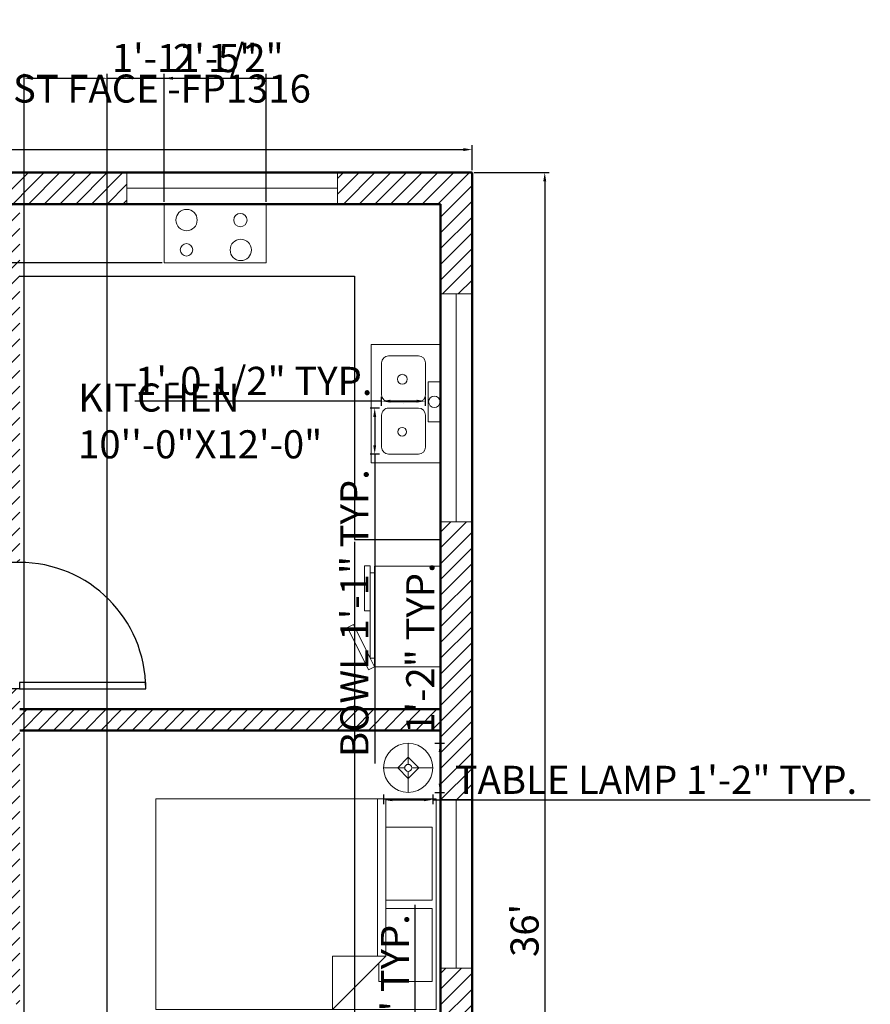
# Model space of a CAD drawing. Units: inches. Extents: x 1188 to 1681, y 1982 to 2608.
# Tile 4 of 4: x 1439 to 1681, y 2259 to 2540. Entities that reach past the tile are written whole.
import ezdxf

# ---------------------------------------------------------------- set-up
doc = ezdxf.new("R2010")
doc.units = ezdxf.units.IN
for name, color, linetype, lineweight in [('A-ANNO-DIMS', 2, 'Continuous', 18), ('A-ANNO-TEXT', 7, 'Continuous', 25), ('A-AREA-IDEN', 7, 'Continuous', 18), ('A-DOOR', 4, 'Continuous', 25), ('A-EQPM', 9, 'Continuous', 20), ('A-FLOR-CASE', 8, 'Continuous', 25), ('A-FLOR-FIXT', 9, 'Continuous', 18), ('A-FURN', 8, 'Continuous', 18), ('A-GLAZ', 4, 'Continuous', 20), ('A-WALL', 7, 'Continuous', 50), ('A-WALL-PATT', 8, 'Continuous', 13)]:
    doc.layers.add(name, color=color, linetype=linetype, lineweight=lineweight)
doc.styles.get("Standard").update_dxf_attribs({"font": 'arial.ttf'})
doc.dimstyles.new('ISO-25', dxfattribs={"dimtxt": 8, "dimasz": 2.5, "dimexe": 1.25, "dimexo": 0.625, "dimtad": 1, "dimdec": 1, "dimlunit": 4, "dimtxsty": 'Standard', "dimcen": 2.5, "dimadec": 0, "dimazin": 0, "dimtfac": 1, "dimtdec": 1, "dimtmove": 0, "dimatfit": 3, "dimfxl": 1, "dimarcsym": 0})

# ---------------------------------------------------------------- blocks, each defined once
blk = doc.blocks.new('*U5')
for p, q in [((0, 0), (0, 6)), ((36, 0), (36, 6))]:
    blk.add_line(p, q)
blk.add_lwpolyline([(0, 0), (0, -36), (1.75, -36), (1.75, 0)], close=True)
blk.add_arc((0, 0), 36, 270, 0)
blk = doc.blocks.new('Lamp - Table')
for p, q in [((0, 7), (0, 1)), ((0, 3), (-3, 0)), ((3, 0), (0, 3)), ((-1, 0), (-7, 0)), ((-3, 0), (0, -3)), ((0, -3), (3, 0)), ((1, 0), (7, 0)), ((0, -1), (0, -7))]:
    blk.add_line(p, q)
for radius in [7, 1]:
    blk.add_circle((0, 0), radius)
blk = doc.blocks.new('Bed - Queen')
for p, q in [((0, -80.00003), (0, 0)), ((0, 0), (59.99999, 0)), ((59.99999, 0), (59.99999, -80.00003)), ((7.99999, -1.2), (28.79998, -1.2)), ((7.99999, -14.4), (7.99999, -1.2)), ((28.79998, -1.2), (28.79998, -14.4)), ((31.19999, -1.2), (51.99999, -1.2)), ((31.19999, -14.4), (31.19999, -1.2)), ((51.99999, -1.2), (51.99999, -16.4)), ((0, -14.4), (44.8, -14.4)), ((44.8, -16.8), (0, -16.8)), ((59.99999, -29.6), (44.8, -14.4)), ((44.8, -14.4), (44.8, -29.6)), ((51.99999, -16.4), (46.79936, -16.4)), ((44.8, -29.6), (59.99999, -29.6)), ((59.99999, -80.00003), (0, -80.00003))]:
    blk.add_line(p, q)
blk = doc.blocks.new('*D13')
at = {"layer": 'A-ANNO-DIMS', "color": 0, "lineweight": -2, "transparency": 16777216}
for p, q in [((1568.34, 2496.41), (1589.68, 2496.41)), ((1588.43, 2493.91), (1588.43, 2066.91)), ((1568.34, 2064.41), (1589.68, 2064.41))]:
    blk.add_line(p, q, dxfattribs=at)
at = {"layer": 'A-ANNO-DIMS', "color": 0, "transparency": 16777216}
for points in [[(1588.02, 2493.91), (1588.85, 2493.91), (1588.43, 2496.41)], [(1588.02, 2066.91), (1588.85, 2066.91), (1588.43, 2064.41)]]:
    blk.add_solid(points, dxfattribs=at)
at = {"layer": 'Defpoints', "color": 0, "transparency": 16777216}
for p in [(1567.72, 2496.41), (1567.72, 2064.41), (1588.43, 2064.41)]:
    blk.add_point(p, dxfattribs=at)
at = {"layer": 'A-ANNO-DIMS', "color": 0, "transparency": 16777216, "insert": (1583.72, 2280.41), "char_height": 8, "attachment_point": 5, "rotation": 90}
blk.add_mtext("36'", dxfattribs=at)
blk = doc.blocks.new('*D14')
at = {"layer": 'A-ANNO-DIMS', "color": 0, "lineweight": -2, "transparency": 16777216}
for p, q in [((1231.72, 2497.04), (1231.72, 2504.18)), ((1567.72, 2497.04), (1567.72, 2504.18)), ((1234.22, 2502.93), (1565.22, 2502.93))]:
    blk.add_line(p, q, dxfattribs=at)
at = {"layer": 'A-ANNO-DIMS', "color": 0, "transparency": 16777216}
for points in [[(1234.22, 2503.35), (1234.22, 2502.52), (1231.72, 2502.93)], [(1565.22, 2503.35), (1565.22, 2502.52), (1567.72, 2502.93)]]:
    blk.add_solid(points, dxfattribs=at)
at = {"layer": 'Defpoints', "color": 0, "transparency": 16777216}
for p in [(1567.72, 2502.93), (1231.72, 2496.41), (1567.72, 2496.41)]:
    blk.add_point(p, dxfattribs=at)
at = {"layer": 'A-ANNO-DIMS', "color": 0, "transparency": 16777216, "insert": (1399.72, 2507.64), "char_height": 8, "attachment_point": 5}
blk.add_mtext("28'", dxfattribs=at)
blk = doc.blocks.new('WIN-60IN')
for p, q in [((0, 9), (0, 0)), ((60, 0), (60, 9)), ((60, 9), (60, 4.5)), ((60, 4.5), (0, 4.5)), ((0, 0), (60, 0))]:
    blk.add_line(p, q)
blk = doc.blocks.new('WIN-48IN')
for p, q in [((0, 9), (0, 0)), ((48, 0), (48, 9)), ((48, 9), (48, 4.5)), ((48, 4.5), (0, 4.5)), ((0, 0), (48, 0))]:
    blk.add_line(p, q)
blk = doc.blocks.new('SINK-BOWL')
for p, q in [((10.48, 13.11), (2, 13.11)), ((0, 11.11), (0, 2)), ((12.48, 2), (12.48, 11.11)), ((2, 0), (10.48, 0))]:
    blk.add_line(p, q)
for centre, start, end in [((2, 11.11), 90, 180), ((10.48, 11.11), 0, 90), ((2, 2), 180, 270), ((10.48, 2), 270, 0)]:
    blk.add_arc(centre, 2, start, end)
blk = doc.blocks.new('*D22')
at = {"layer": 'A-ANNO-DIMS', "color": 0, "lineweight": -2, "transparency": 16777216}
for p, q in [((1542.5, 2319.11), (1542.5, 2316.38)), ((1556.5, 2319.11), (1556.5, 2316.38)), ((1545, 2317.63), (1554, 2317.63)), ((1556.5, 2317.63), (1681.27, 2317.63))]:
    blk.add_line(p, q, dxfattribs=at)
at = {"layer": 'A-ANNO-DIMS', "color": 0, "transparency": 16777216}
for points in [[(1545, 2318.05), (1545, 2317.22), (1542.5, 2317.63)], [(1554, 2318.05), (1554, 2317.22), (1556.5, 2317.63)]]:
    blk.add_solid(points, dxfattribs=at)
at = {"layer": 'Defpoints', "color": 0, "transparency": 16777216}
for p in [(1542.5, 2319.73), (1556.5, 2319.73), (1556.5, 2317.63)]:
    blk.add_point(p, dxfattribs=at)
at = {"layer": 'A-ANNO-DIMS', "color": 0, "transparency": 16777216, "insert": (1620.14, 2322.28), "char_height": 8, "attachment_point": 5}
blk.add_mtext('TABLE LAMP 1\'-2" TYP.', dxfattribs=at)
blk = doc.blocks.new('*D23')
at = {"layer": 'A-ANNO-DIMS', "color": 0, "lineweight": -2, "transparency": 16777216}
for p, q in [((1558.6, 2333.73), (1558.6, 2385.5)), ((1557.13, 2333.73), (1559.85, 2333.73)), ((1558.6, 2322.23), (1558.6, 2331.23)), ((1557.13, 2319.73), (1559.85, 2319.73))]:
    blk.add_line(p, q, dxfattribs=at)
at = {"layer": 'A-ANNO-DIMS', "color": 0, "transparency": 16777216}
for points in [[(1558.19, 2331.23), (1559.02, 2331.23), (1558.6, 2333.73)], [(1558.19, 2322.23), (1559.02, 2322.23), (1558.6, 2319.73)]]:
    blk.add_solid(points, dxfattribs=at)
at = {"layer": 'Defpoints', "color": 0, "transparency": 16777216}
for p in [(1556.5, 2333.73), (1558.6, 2333.73), (1556.5, 2319.73)]:
    blk.add_point(p, dxfattribs=at)
at = {"layer": 'A-ANNO-DIMS', "color": 0, "transparency": 16777216, "insert": (1553.96, 2360.87), "char_height": 8, "attachment_point": 5, "rotation": 90}
blk.add_mtext('1\'-2" TYP.', dxfattribs=at)
blk = doc.blocks.new('*D26')
at = {"layer": 'A-ANNO-DIMS', "color": 0, "lineweight": -2, "transparency": 16777216}
for p, q in [((1551.52, 2182.72), (1551.52, 2287.7)), ((1558.09, 2182.72), (1550.27, 2182.72)), ((1551.52, 2137.22), (1551.52, 2180.22)), ((1558.09, 2134.72), (1550.27, 2134.72))]:
    blk.add_line(p, q, dxfattribs=at)
at = {"layer": 'A-ANNO-DIMS', "color": 0, "transparency": 16777216}
for points in [[(1551.1, 2180.22), (1551.93, 2180.22), (1551.52, 2182.72)], [(1551.1, 2137.22), (1551.93, 2137.22), (1551.52, 2134.72)]]:
    blk.add_solid(points, dxfattribs=at)
at = {"layer": 'Defpoints', "color": 0, "transparency": 16777216}
for p in [(1551.52, 2182.72), (1558.72, 2182.72), (1558.72, 2134.72)]:
    blk.add_point(p, dxfattribs=at)
at = {"layer": 'A-ANNO-DIMS', "color": 0, "transparency": 16777216, "insert": (1546.75, 2236.46), "char_height": 8, "attachment_point": 5, "rotation": 90}
blk.add_mtext('WINDOW 4\'-0" TYP.', dxfattribs=at)
blk = doc.blocks.new('*D36')
at = {"layer": 'A-ANNO-DIMS', "color": 0, "lineweight": -2, "transparency": 16777216}
for p, q in [((1541.29, 2429.27), (1538.7, 2429.27)), ((1539.95, 2426.77), (1539.95, 2418.66)), ((1541.29, 2416.16), (1538.7, 2416.16)), ((1539.95, 2416.16), (1539.95, 2327.98))]:
    blk.add_line(p, q, dxfattribs=at)
at = {"layer": 'A-ANNO-DIMS', "color": 0, "transparency": 16777216}
for points in [[(1539.54, 2426.77), (1540.37, 2426.77), (1539.95, 2429.27)], [(1539.54, 2418.66), (1540.37, 2418.66), (1539.95, 2416.16)]]:
    blk.add_solid(points, dxfattribs=at)
at = {"layer": 'Defpoints', "color": 0, "transparency": 16777216}
for p in [(1541.92, 2429.27), (1539.95, 2416.16), (1541.92, 2416.16)]:
    blk.add_point(p, dxfattribs=at)
at = {"layer": 'A-ANNO-DIMS', "color": 0, "transparency": 16777216, "insert": (1535.19, 2370.82), "char_height": 8, "attachment_point": 5, "rotation": 90}
blk.add_mtext('BOWL 1\'-1" TYP.', dxfattribs=at)
blk = doc.blocks.new('*D37')
at = {"layer": 'A-ANNO-DIMS', "color": 0, "lineweight": -2, "transparency": 16777216}
for p, q in [((1541.92, 2431.23), (1471.52, 2431.23)), ((1541.92, 2429.89), (1541.92, 2432.48)), ((1551.9, 2431.23), (1544.42, 2431.23)), ((1554.4, 2429.89), (1554.4, 2432.48))]:
    blk.add_line(p, q, dxfattribs=at)
at = {"layer": 'A-ANNO-DIMS', "color": 0, "transparency": 16777216}
for points in [[(1544.42, 2431.65), (1544.42, 2430.82), (1541.92, 2431.23)], [(1551.9, 2431.65), (1551.9, 2430.82), (1554.4, 2431.23)]]:
    blk.add_solid(points, dxfattribs=at)
at = {"layer": 'Defpoints', "color": 0, "transparency": 16777216}
for p in [(1541.92, 2431.23), (1541.92, 2429.27), (1554.4, 2429.27)]:
    blk.add_point(p, dxfattribs=at)
at = {"layer": 'A-ANNO-DIMS', "color": 0, "transparency": 16777216, "insert": (1505.47, 2435.99), "char_height": 8, "attachment_point": 5}
blk.add_mtext('1\'-0 1/2" TYP.', dxfattribs=at)
blk = doc.blocks.new('*D52')
at = {"layer": 'A-ANNO-DIMS', "color": 0, "lineweight": -2, "transparency": 16777216}
for p, q in [((1534.2, 2391.18), (1534.2, 1988.31)), ((1558.72, 2391.18), (1558.72, 1988.31)), ((1534.2, 1989.56), (1490.41, 1989.56)), ((1556.22, 1989.56), (1536.7, 1989.56))]:
    blk.add_line(p, q, dxfattribs=at)
at = {"layer": 'A-ANNO-DIMS', "color": 0, "transparency": 16777216}
for points in [[(1536.7, 1989.98), (1536.7, 1989.15), (1534.2, 1989.56)], [(1556.22, 1989.98), (1556.22, 1989.15), (1558.72, 1989.56)]]:
    blk.add_solid(points, dxfattribs=at)
at = {"layer": 'Defpoints', "color": 0, "transparency": 16777216}
for p in [(1534.2, 2391.81), (1558.72, 2391.81), (1534.2, 1989.56)]:
    blk.add_point(p, dxfattribs=at)
at = {"layer": 'A-ANNO-DIMS', "color": 0, "transparency": 16777216, "insert": (1511.06, 1994.33), "char_height": 8, "attachment_point": 5}
blk.add_mtext('2\'-0 1/2"', dxfattribs=at)
blk = doc.blocks.new('*D53')
at = {"layer": 'A-ANNO-DIMS', "color": 0, "lineweight": -2, "transparency": 16777216}
for p, q in [((1479.94, 2488.04), (1479.94, 2524.51)), ((1482.44, 2523.26), (1506.5, 2523.26)), ((1509, 2488.04), (1509, 2524.51))]:
    blk.add_line(p, q, dxfattribs=at)
at = {"layer": 'A-ANNO-DIMS', "color": 0, "transparency": 16777216}
for points in [[(1482.44, 2523.68), (1482.44, 2522.85), (1479.94, 2523.26)], [(1506.5, 2523.68), (1506.5, 2522.85), (1509, 2523.26)]]:
    blk.add_solid(points, dxfattribs=at)
at = {"layer": 'Defpoints', "color": 0, "transparency": 16777216}
for p in [(1509, 2523.26), (1479.94, 2487.41), (1509, 2487.41)]:
    blk.add_point(p, dxfattribs=at)
at = {"layer": 'A-ANNO-DIMS', "color": 0, "transparency": 16777216, "insert": (1494.47, 2527.97), "char_height": 8, "attachment_point": 5}
blk.add_mtext('2\'-5"', dxfattribs=at)
blk = doc.blocks.new('*D54')
at = {"layer": 'A-ANNO-DIMS', "color": 0, "lineweight": -2, "transparency": 16777216}
for p, q in [((1479.32, 2487.41), (1203.62, 2487.41)), ((1204.87, 2484.91), (1204.87, 2473.18)), ((1479.32, 2470.68), (1203.62, 2470.68)), ((1204.87, 2470.68), (1204.87, 2427.77))]:
    blk.add_line(p, q, dxfattribs=at)
at = {"layer": 'A-ANNO-DIMS', "color": 0, "transparency": 16777216}
for points in [[(1204.45, 2484.91), (1205.28, 2484.91), (1204.87, 2487.41)], [(1204.45, 2473.18), (1205.28, 2473.18), (1204.87, 2470.68)]]:
    blk.add_solid(points, dxfattribs=at)
at = {"layer": 'Defpoints', "color": 0, "transparency": 16777216}
for p in [(1479.94, 2487.41), (1204.87, 2470.68), (1479.94, 2470.68)]:
    blk.add_point(p, dxfattribs=at)
at = {"layer": 'A-ANNO-DIMS', "color": 0, "transparency": 16777216, "insert": (1200.11, 2447.98), "char_height": 8, "attachment_point": 5, "rotation": 90}
blk.add_mtext('1\'-4 1/2"', dxfattribs=at)
blk = doc.blocks.new('*D57')
at = {"layer": 'A-ANNO-DIMS', "color": 0, "lineweight": -2, "transparency": 16777216}
for p, q in [((1440.02, 2125.93), (1440.02, 2524.51)), ((1442.52, 2523.26), (1461.18, 2523.26)), ((1463.68, 2125.93), (1463.68, 2524.51)), ((1463.68, 2523.26), (1512.8, 2523.26))]:
    blk.add_line(p, q, dxfattribs=at)
at = {"layer": 'A-ANNO-DIMS', "color": 0, "transparency": 16777216}
for points in [[(1442.52, 2523.68), (1442.52, 2522.85), (1440.02, 2523.26)], [(1461.18, 2523.68), (1461.18, 2522.85), (1463.68, 2523.26)]]:
    blk.add_solid(points, dxfattribs=at)
at = {"layer": 'Defpoints', "color": 0, "transparency": 16777216}
for p in [(1463.68, 2523.26), (1440.02, 2125.31), (1463.68, 2125.31)]:
    blk.add_point(p, dxfattribs=at)
at = {"layer": 'A-ANNO-DIMS', "color": 0, "transparency": 16777216, "insert": (1489.49, 2528.03), "char_height": 8, "attachment_point": 5}
blk.add_mtext('1\'-11 1/2"', dxfattribs=at)

msp = doc.modelspace()

# ---------------------------------------------------------------- hatches: boundary and pattern name
at = {"layer": 'A-WALL-PATT', "transparency": 33554559}
h = msp.add_hatch(dxfattribs=at)
h.set_pattern_fill('ANSI31', color=256)
h.paths.add_polyline_path([(1390.99, 2496.41), (1231.72, 2496.41), (1231.72, 2452.82), (1240.72, 2452.82), (1240.72, 2487.41), (1390.99, 2487.41)])
h.paths.add_polyline_path([(1469.3, 2496.41), (1426.99, 2496.41), (1426.99, 2491.91), (1426.99, 2487.41), (1469.3, 2487.41)])
h.paths.add_polyline_path([(1378.72, 2487.41), (1372.72, 2487.41), (1372.72, 2404.84), (1372.72, 2343.41), (1367.48, 2343.41), (1367.48, 2337.41), (1378.72, 2337.41), (1378.72, 2391.41), (1387.67, 2391.41), (1387.67, 2397.41), (1378.72, 2397.41)])
h.paths.add_polyline_path([(1438.72, 2487.41), (1432.72, 2487.41), (1432.72, 2397.41), (1420.72, 2397.41), (1420.72, 2391.41), (1432.72, 2391.41), (1432.72, 2385.41), (1438.72, 2385.41)])
h.paths.add_polyline_path([(1240.72, 2392.82), (1236.22, 2392.82), (1231.72, 2392.82), (1231.72, 2323.77), (1240.72, 2323.77)])
h.paths.add_polyline_path([(1330.72, 2343.41), (1240.72, 2343.41), (1240.72, 2337.41), (1330.72, 2337.41)])
h.paths.add_polyline_path([(1558.72, 2343.41), (1438.72, 2343.41), (1438.72, 2349.29), (1438.64, 2349.29), (1432.72, 2349.29), (1432.72, 2259.41), (1438.72, 2259.41), (1438.72, 2337.41), (1558.72, 2337.41)])
h.paths.add_polyline_path([(1567.72, 2396.81), (1558.72, 2396.81), (1558.72, 2317.68), (1563.22, 2317.68), (1567.72, 2317.68)])
h.paths.add_polyline_path([(1567.72, 2496.41), (1529.3, 2496.41), (1529.3, 2491.91), (1529.3, 2487.41), (1558.72, 2487.41), (1558.72, 2461.81), (1567.72, 2461.81)])
h.paths.add_polyline_path([(1240.72, 2195.41), (1240.72, 2201.41), (1240.72, 2263.77), (1231.72, 2263.77), (1231.72, 2016.41), (1246.72, 2016.41), (1246.72, 2022.41), (1246.72, 2025.41), (1240.72, 2025.41)])
h.paths.add_polyline_path([(1391.72, 2211.41), (1397.72, 2211.41), (1397.72, 2217.41), (1385.72, 2217.41), (1385.72, 2163.41), (1366.72, 2163.41), (1366.72, 2157.41), (1385.72, 2157.41), (1385.72, 2073.41), (1391.72, 2073.41)])
h.paths.add_polyline_path([(1330.72, 2201.41), (1282.72, 2201.41), (1282.72, 2195.41), (1324.72, 2195.41), (1324.72, 2064.41), (1345.75, 2064.41), (1345.75, 2073.41), (1330.72, 2073.41), (1330.72, 2157.41), (1336.72, 2157.41), (1336.72, 2163.41), (1330.72, 2163.41)])
h.paths.add_polyline_path([(1558.72, 2217.41), (1438.72, 2217.41), (1438.72, 2223.26), (1432.72, 2223.26), (1432.72, 2217.41), (1427.72, 2217.41), (1427.72, 2211.41), (1432.72, 2211.41), (1558.72, 2211.41)])
h.paths.add_polyline_path([(1567.72, 2269.68), (1558.72, 2269.68), (1558.72, 2182.72), (1563.22, 2182.72), (1567.72, 2182.72)])
h.paths.add_polyline_path([(1567.72, 2134.72), (1558.72, 2134.72), (1558.72, 2073.41), (1497.85, 2073.41), (1497.85, 2068.91), (1497.85, 2064.41), (1567.72, 2064.41)])
h.paths.add_polyline_path([(1449.85, 2073.41), (1371.31, 2073.41), (1371.31, 2068.91), (1371.31, 2064.41), (1449.85, 2064.41)])
h.paths.add_polyline_path([(1333.72, 2064.41), (1324.72, 2064.41), (1324.72, 2025.41), (1313.9, 2025.41), (1313.9, 2016.41), (1333.72, 2016.41)])

# ---------------------------------------------------------------- linework, layer by layer
at = {"layer": 'A-EQPM'}
for p, q in [((1479.94, 2487.41), (1479.94, 2470.68)), ((1509, 2470.68), (1509, 2487.41)), ((1479.94, 2470.68), (1509, 2470.68)), ((1538.68, 2384.3), (1537, 2384.3)), ((1537, 2384.3), (1537, 2371.52)), ((1538.68, 2382.28), (1538.68, 2384.3)), ((1558.72, 2384.25), (1539.9, 2384.25)), ((1539.9, 2384.25), (1539.9, 2355.54)), ((1539.9, 2382.28), (1538.68, 2382.28)), ((1538.68, 2382.28), (1538.68, 2358.01)), ((1537, 2371.52), (1538.68, 2371.52)), ((1532.23, 2366.7), (1533.94, 2367.55)), ((1538.19, 2354.69), (1532.23, 2366.7)), ((1533.94, 2367.55), (1538.68, 2358.01)), ((1538.68, 2358.01), (1539.9, 2358.01)), ((1538.68, 2358.01), (1539.9, 2355.54)), ((1539.9, 2355.54), (1538.19, 2354.69)), ((1539.9, 2355.54), (1558.72, 2355.54))]:
    msp.add_line(p, q, dxfattribs=at)
for centre, radius in [((1486.29, 2482.85), 3.04), ((1501.64, 2482.85), 1.9), ((1486.29, 2474.35), 1.78), ((1501.77, 2474.35), 3.04)]:
    msp.add_circle(centre, radius, dxfattribs=at)
at = {"layer": 'A-FLOR-CASE'}
for p, q in [((1438.72, 2466.87), (1438.72, 2466.87)), ((1438.72, 2466.87), (1534.2, 2466.87)), ((1534.2, 2466.87), (1534.2, 2391.81)), ((1534.2, 2391.81), (1558.72, 2391.81))]:
    msp.add_line(p, q, dxfattribs=at)
at = {"layer": 'A-FLOR-FIXT'}
msp.add_line((1548.28, 2430.45), (1548.28, 2430.45), dxfattribs=at)
for points in [[(1558.72, 2447.35), (1538.96, 2447.35), (1538.96, 2413.68), (1558.72, 2413.68)], [(1555.18, 2436.76), (1558.72, 2436.76), (1558.72, 2425.38), (1555.18, 2425.38)]]:
    msp.add_lwpolyline(points, close=True, dxfattribs=at)
for centre, radius in [((1547.83, 2437.49), 1.4), ((1556.95, 2431.07), 1.63), ((1547.75, 2422.53), 1.23)]:
    msp.add_circle(centre, radius, dxfattribs=at)
at = {"layer": 'A-GLAZ'}
for p, q in [((1558.72, 2461.81), (1567.72, 2461.81)), ((1563.22, 2396.81), (1563.22, 2461.81)), ((1567.72, 2461.81), (1567.72, 2456.81)), ((1567.72, 2456.81), (1567.72, 2396.81)), ((1567.72, 2396.81), (1558.72, 2396.81)), ((1558.72, 2396.81), (1563.22, 2396.81))]:
    msp.add_line(p, q, dxfattribs=at)
at = {"layer": 'A-WALL'}
for p, q in [((1231.72, 2496.41), (1567.72, 2496.41)), ((1567.72, 2496.41), (1567.72, 2016.41)), ((1240.72, 2487.41), (1558.72, 2487.41)), ((1558.72, 2487.41), (1558.72, 2073.41)), ((1438.72, 2343.41), (1558.72, 2343.41)), ((1438.72, 2337.41), (1558.72, 2337.41))]:
    msp.add_line(p, q, dxfattribs=at)

# ---------------------------------------------------------------- block references
at = {"layer": 'A-DOOR', "rotation": 90}
msp.add_blockref('*U5', (1438.64, 2349.29), dxfattribs=at)
at = {"layer": 'A-FLOR-FIXT'}
msp.add_blockref('SINK-BOWL', (1541.92, 2431.05), dxfattribs=at)
at = {"layer": 'A-FLOR-FIXT', "rotation": 180}
msp.add_blockref('SINK-BOWL', (1554.4, 2429.27), dxfattribs=at)
at = {"layer": 'A-FURN'}
msp.add_blockref('Lamp - Table', (1549.5, 2326.73), dxfattribs=at)
at = {"layer": 'A-FURN', "rotation": 270}
msp.add_blockref('Bed - Queen', (1557.52, 2317.86), dxfattribs=at)
at = {"layer": 'A-GLAZ'}
msp.add_blockref('WIN-60IN', (1469.3, 2487.41), dxfattribs=at)
at = {"layer": 'A-GLAZ', "rotation": 89.99999999999909}
msp.add_blockref('WIN-48IN', (1567.72, 2269.68), dxfattribs=at)

# ---------------------------------------------------------------- texts
at = {"layer": 'A-ANNO-TEXT', "insert": (1239.94, 2524.33), "char_height": 8, "attachment_point": 1}
msp.add_mtext('28X40 (1120 SQ FT) HOUSSE PLAN - WEST FACE -FP1316', dxfattribs=at)
at = {"layer": 'A-AREA-IDEN', "insert": (1455.38, 2436.27), "char_height": 8, "attachment_point": 1}
msp.add_mtext('KITCHEN\\P10\'\'-0"X12\'-0"', dxfattribs=at)

# ---------------------------------------------------------------- dimensions: what is measured, and where the dimension line sits
at = {"layer": 'A-ANNO-DIMS'}
for base, p1, p2, override, picture, middle in [((1463.68, 2523.26), (1440.02, 2125.31), (1463.68, 2125.31), {"dimdec": 1, "dimlfac": 1, "dimrnd": 0, "dimzin": 1, "dimdsep": 46, "dimlunit": 4, "dimfrac": 2}, '*D57', (1489.49, 2528.03)), ((1509, 2523.26), (1479.94, 2487.41), (1509, 2487.41), {"dimdec": 1, "dimlfac": 1, "dimrnd": 0, "dimzin": 1, "dimdsep": 46, "dimlunit": 4, "dimfrac": 2}, '*D53', (1494.47, 2527.97)), ((1567.72, 2502.93), (1231.72, 2496.41), (1567.72, 2496.41), {"dimclrd": 0, "dimclre": 0, "dimclrt": 0}, '*D14', (1399.72, 2507.64)), ((1534.2, 1989.56), (1558.72, 2391.81), (1534.2, 2391.81), {"dimdec": 1, "dimlfac": 1, "dimrnd": 0, "dimzin": 1, "dimdsep": 46, "dimlunit": 4, "dimfrac": 2}, '*D52', (1511.06, 1994.33))]:
    dim = msp.add_linear_dim(base=base, p1=p1, p2=p2, dimstyle='ISO-25', override=override, dxfattribs=at)
    dim.commit()
    dim.dimension.update_dxf_attribs({"geometry": picture, "text_midpoint": middle})
for base, p1, p2, override, picture, middle in [((1588.43, 2064.41), (1567.72, 2496.41), (1567.72, 2064.41), {"dimclrd": 0, "dimclre": 0, "dimclrt": 0}, '*D13', (1583.72, 2280.41)), ((1204.87, 2470.68), (1479.94, 2487.41), (1479.94, 2470.68), {"dimdec": 1, "dimlfac": 1, "dimrnd": 0, "dimzin": 1, "dimdsep": 46, "dimlunit": 4, "dimfrac": 2}, '*D54', (1200.11, 2447.98))]:
    dim = msp.add_linear_dim(base=base, p1=p1, p2=p2, angle=90, dimstyle='ISO-25', override=override, dxfattribs=at)
    dim.commit()
    dim.dimension.update_dxf_attribs({"geometry": picture, "text_midpoint": middle})
for base, p1, p2, angle, text, picture, middle in [((1541.92, 2431.23), (1554.4, 2429.27), (1541.92, 2429.27), 180, '<> TYP.', '*D37', (1505.47, 2435.99)), ((1539.95, 2416.16), (1541.92, 2429.27), (1541.92, 2416.16), 270, 'BOWL <> TYP.', '*D36', (1535.19, 2370.82)), ((1558.6, 2333.73), (1556.5, 2319.73), (1556.5, 2333.73), 90, '<> TYP.', '*D23', (1553.96, 2360.87)), ((1551.52, 2182.72), (1558.72, 2134.72), (1558.72, 2182.72), 90, 'WINDOW <> TYP.', '*D26', (1546.75, 2236.46))]:
    dim = msp.add_linear_dim(base=base, p1=p1, p2=p2, angle=angle, text=text, dimstyle='ISO-25', override={"dimdec": 1, "dimlfac": 1, "dimrnd": 0, "dimzin": 1, "dimdsep": 46, "dimlunit": 4, "dimfrac": 2}, dxfattribs=at)
    dim.commit()
    dim.dimension.update_dxf_attribs({"geometry": picture, "text_midpoint": middle})
dim = msp.add_linear_dim(base=(1556.5, 2317.63), p1=(1542.5, 2319.73), p2=(1556.5, 2319.73), text='TABLE LAMP <> TYP.', dimstyle='ISO-25', override={"dimdec": 1, "dimlfac": 1, "dimrnd": 0, "dimzin": 1, "dimdsep": 46, "dimlunit": 4, "dimfrac": 2}, dxfattribs=at)
dim.commit()
dim.dimension.update_dxf_attribs({"geometry": '*D22', "text_midpoint": (1620.14, 2322.28)})

doc.saveas('drawing.dxf')
